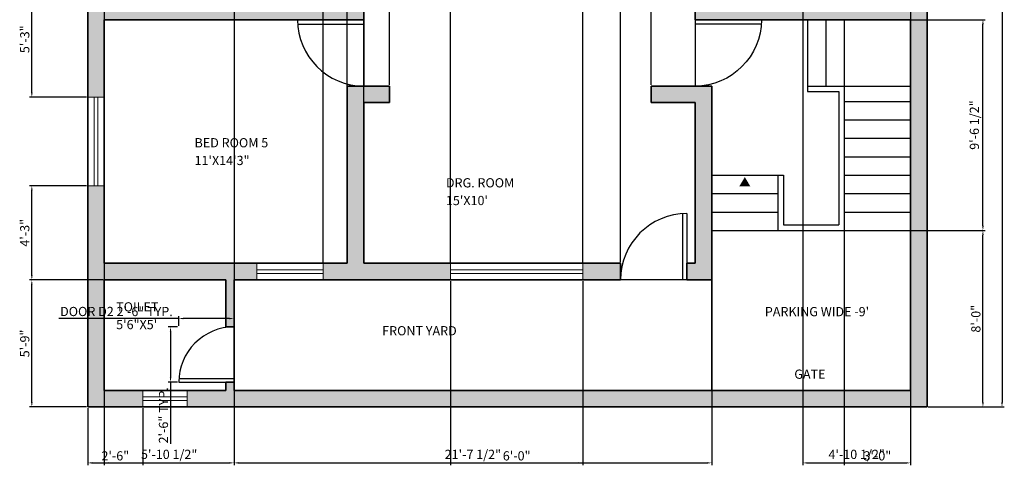
# Model space of a CAD drawing. Units: inches. Extents: x 2263 to 2802, y 2658 to 3310.
# Tile 1 of 3: x 2267 to 2802, y 2658 to 2902. Entities that reach past the tile are written whole.
import ezdxf

# ---------------------------------------------------------------- set-up
doc = ezdxf.new("R2010")
doc.units = ezdxf.units.IN
doc.header["$LTSCALE"] = 0.3
for name, color, linetype, lineweight in [('A-ANNO-DIMS', 2, 'Continuous', 18), ('A-ANNO-TEXT', 7, 'Continuous', 18), ('A-AREA-IDEN', 7, 'Continuous', 18), ('A-DOOR', 3, 'Continuous', 25), ('A-FLOR-STRS', 7, 'Continuous', 25), ('A-GLAZ', 4, 'Continuous', 18), ('A-WALL', 7, 'Continuous', 35)]:
    doc.layers.add(name, color=color, linetype=linetype, lineweight=lineweight)
doc.layers.add('A-WALL-PATT', color=18, linetype='Continuous', lineweight=13, true_color=0x000000)
doc.styles.get("Standard").update_dxf_attribs({"font": 'calibri.ttf', "height": 5})
doc.dimstyles.new('ISO-25', dxfattribs={"dimtxt": 5, "dimasz": 2.5, "dimexe": 1.25, "dimexo": 0.625, "dimtad": 1, "dimlunit": 3, "dimtxsty": 'Standard', "dimcen": 2.5, "dimadec": 0, "dimazin": 0, "dimtfac": 1, "dimtmove": 0, "dimatfit": 3, "dimfxl": 1, "dimarcsym": 0})

# ---------------------------------------------------------------- blocks, each defined once
blk = doc.blocks.new('*D2')
at = {"layer": 'A-ANNO-DIMS', "color": 0, "lineweight": -2, "transparency": 16777216}
for p, q in [((2761.03, 3268.27), (2802.38, 3268.27)), ((2801.13, 3265.77), (2801.13, 2694.77)), ((2761.03, 2692.27), (2802.38, 2692.27))]:
    blk.add_line(p, q, dxfattribs=at)
at = {"layer": 'A-ANNO-DIMS', "color": 0, "lineweight": -3, "transparency": 16777216}
for points in [[(2800.71, 3265.77), (2801.54, 3265.77), (2801.13, 3268.27)], [(2800.71, 2694.77), (2801.54, 2694.77), (2801.13, 2692.27)]]:
    blk.add_solid(points, dxfattribs=at)
at = {"layer": 'Defpoints', "color": 0, "lineweight": -3, "transparency": 16777216}
for p in [(2760.41, 3268.27), (2760.41, 2692.27), (2801.13, 2692.27)]:
    blk.add_point(p, dxfattribs=at)
at = {"layer": 'A-ANNO-DIMS', "color": 0, "transparency": 16777216, "insert": (2797.94, 2980.27), "char_height": 5, "attachment_point": 5, "rotation": 90}
blk.add_mtext("48'", dxfattribs=at)
blk = doc.blocks.new('DOOR-SWING-36')
for p, q in [((0, 0), (0, 36)), ((35.92, 2.4), (0, 2.4)), ((36, 0), (0, 0))]:
    blk.add_line(p, q)
blk.add_arc((0, 0), 36, 0, 90)
blk = doc.blocks.new('DOOR-SWING-30')
for p, q in [((30, 0), (0, 0)), ((0, 0), (0, -30)), ((29.93, -2), (0, -2))]:
    blk.add_line(p, q)
blk.add_arc((0, 0), 30, 270, 0)
blk = doc.blocks.new('WIN-24')
for p, q in [((0, 0), (0, -24)), ((9, 0), (0, 0)), ((3.5, 0), (3.5, -24)), ((5.5, 0), (5.5, -24)), ((9, -24), (9, 0)), ((0, -24), (9, -24))]:
    blk.add_line(p, q)
blk = doc.blocks.new('WIN-36')
for p, q in [((0, 36), (-9, 36)), ((-9, 36), (-9, 0)), ((-5.5, 0), (-5.5, 36)), ((-3.5, 0), (-3.5, 36)), ((0, 0), (0, 36)), ((-9, 0), (0, 0))]:
    blk.add_line(p, q)
blk = doc.blocks.new('WIN-48')
for p, q in [((0, 48), (-9, 48)), ((-9, 48), (-9, 0)), ((-5.5, 0), (-5.5, 48)), ((-3.5, 0), (-3.5, 48)), ((0, 0), (0, 48)), ((-9, 0), (0, 0))]:
    blk.add_line(p, q)
blk = doc.blocks.new('*D11')
at = {"layer": 'A-ANNO-DIMS', "color": 0, "lineweight": -2, "transparency": 16777216}
for p, q in [((2353.91, 2740.27), (2288.64, 2740.27)), ((2353.91, 2736.4), (2353.91, 2741.52)), ((2381.41, 2740.27), (2356.41, 2740.27)), ((2383.91, 2736.4), (2383.91, 2741.52))]:
    blk.add_line(p, q, dxfattribs=at)
at = {"layer": 'A-ANNO-DIMS', "color": 0, "lineweight": -3, "transparency": 16777216}
for points in [[(2356.41, 2740.69), (2356.41, 2739.86), (2353.91, 2740.27)], [(2381.41, 2740.69), (2381.41, 2739.86), (2383.91, 2740.27)]]:
    blk.add_solid(points, dxfattribs=at)
at = {"layer": 'Defpoints', "color": 0, "lineweight": -3, "transparency": 16777216}
for p in [(2353.91, 2740.27), (2353.91, 2735.77), (2383.91, 2735.77)]:
    blk.add_point(p, dxfattribs=at)
at = {"layer": 'A-ANNO-DIMS', "color": 0, "transparency": 16777216, "insert": (2320.02, 2743.46), "char_height": 5, "attachment_point": 5}
blk.add_mtext('DOOR D2 2\'-6" TYP.', dxfattribs=at)
blk = doc.blocks.new('*D12')
at = {"layer": 'A-ANNO-DIMS', "color": 0, "lineweight": -2, "transparency": 16777216}
for p, q in [((2353.28, 2735.77), (2348.16, 2735.77)), ((2349.41, 2733.27), (2349.41, 2708.27)), ((2353.28, 2705.77), (2348.16, 2705.77)), ((2349.41, 2705.77), (2349.41, 2672.23))]:
    blk.add_line(p, q, dxfattribs=at)
at = {"layer": 'A-ANNO-DIMS', "color": 0, "lineweight": -3, "transparency": 16777216}
for points in [[(2348.99, 2733.27), (2349.83, 2733.27), (2349.41, 2735.77)], [(2348.99, 2708.27), (2349.83, 2708.27), (2349.41, 2705.77)]]:
    blk.add_solid(points, dxfattribs=at)
at = {"layer": 'Defpoints', "color": 0, "lineweight": -3, "transparency": 16777216}
for p in [(2353.91, 2735.77), (2349.41, 2705.77), (2353.91, 2705.77)]:
    blk.add_point(p, dxfattribs=at)
at = {"layer": 'A-ANNO-DIMS', "color": 0, "transparency": 16777216, "insert": (2346.22, 2687.75), "char_height": 5, "attachment_point": 5, "rotation": 90}
blk.add_mtext('2\'-6" TYP.', dxfattribs=at)
blk = doc.blocks.new('*D21')
at = {"layer": 'A-ANNO-DIMS', "color": 0, "lineweight": -2, "transparency": 16777216}
for p, q in [((2312.78, 2761.27), (2272.81, 2761.27)), ((2274.06, 2694.77), (2274.06, 2758.77)), ((2303.78, 2692.27), (2272.81, 2692.27))]:
    blk.add_line(p, q, dxfattribs=at)
at = {"layer": 'A-ANNO-DIMS', "color": 0, "lineweight": -3, "transparency": 16777216}
for points in [[(2273.64, 2758.77), (2274.48, 2758.77), (2274.06, 2761.27)], [(2273.64, 2694.77), (2274.48, 2694.77), (2274.06, 2692.27)]]:
    blk.add_solid(points, dxfattribs=at)
at = {"layer": 'Defpoints', "color": 0, "lineweight": -3, "transparency": 16777216}
for p in [(2274.06, 2761.27), (2313.41, 2761.27), (2304.41, 2692.27)]:
    blk.add_point(p, dxfattribs=at)
at = {"layer": 'A-ANNO-DIMS', "color": 0, "transparency": 16777216, "insert": (2270.87, 2726.77), "char_height": 5, "attachment_point": 5, "rotation": 90}
blk.add_mtext('5\'-9"', dxfattribs=at)
blk = doc.blocks.new('*D22')
at = {"layer": 'A-ANNO-DIMS', "color": 0, "lineweight": -2, "transparency": 16777216}
for p, q in [((2303.78, 2812.37), (2272.81, 2812.37)), ((2274.06, 2763.77), (2274.06, 2809.87)), ((2312.78, 2761.27), (2272.81, 2761.27))]:
    blk.add_line(p, q, dxfattribs=at)
at = {"layer": 'A-ANNO-DIMS', "color": 0, "lineweight": -3, "transparency": 16777216}
for points in [[(2273.64, 2809.87), (2274.48, 2809.87), (2274.06, 2812.37)], [(2273.64, 2763.77), (2274.48, 2763.77), (2274.06, 2761.27)]]:
    blk.add_solid(points, dxfattribs=at)
at = {"layer": 'Defpoints', "color": 0, "lineweight": -3, "transparency": 16777216}
for p in [(2274.06, 2812.37), (2304.41, 2812.37), (2313.41, 2761.27)]:
    blk.add_point(p, dxfattribs=at)
at = {"layer": 'A-ANNO-DIMS', "color": 0, "transparency": 16777216, "insert": (2270.87, 2786.82), "char_height": 5, "attachment_point": 5, "rotation": 90}
blk.add_mtext('4\'-3"', dxfattribs=at)
blk = doc.blocks.new('*D23')
at = {"layer": 'A-ANNO-DIMS', "color": 0, "lineweight": -2, "transparency": 16777216}
for p, q in [((2303.78, 2923.37), (2272.81, 2923.37)), ((2274.06, 2862.87), (2274.06, 2920.87)), ((2303.78, 2860.37), (2272.81, 2860.37))]:
    blk.add_line(p, q, dxfattribs=at)
at = {"layer": 'A-ANNO-DIMS', "color": 0, "lineweight": -3, "transparency": 16777216}
for points in [[(2273.64, 2920.87), (2274.48, 2920.87), (2274.06, 2923.37)], [(2273.64, 2862.87), (2274.48, 2862.87), (2274.06, 2860.37)]]:
    blk.add_solid(points, dxfattribs=at)
at = {"layer": 'Defpoints', "color": 0, "lineweight": -3, "transparency": 16777216}
for p in [(2274.06, 2923.37), (2304.41, 2923.37), (2304.41, 2860.37)]:
    blk.add_point(p, dxfattribs=at)
at = {"layer": 'A-ANNO-DIMS', "color": 0, "transparency": 16777216, "insert": (2270.87, 2891.87), "char_height": 5, "attachment_point": 5, "rotation": 90}
blk.add_mtext('5\'-3"', dxfattribs=at)
blk = doc.blocks.new('*D26')
at = {"layer": 'A-ANNO-DIMS', "color": 0, "lineweight": -2, "transparency": 16777216}
for p, q in [((2304.41, 2691.65), (2304.41, 2660.67)), ((2334.41, 2691.65), (2334.41, 2660.67)), ((2306.91, 2661.92), (2331.91, 2661.92))]:
    blk.add_line(p, q, dxfattribs=at)
at = {"layer": 'A-ANNO-DIMS', "color": 0, "lineweight": -3, "transparency": 16777216}
for points in [[(2306.91, 2662.34), (2306.91, 2661.51), (2304.41, 2661.92)], [(2331.91, 2662.34), (2331.91, 2661.51), (2334.41, 2661.92)]]:
    blk.add_solid(points, dxfattribs=at)
at = {"layer": 'Defpoints', "color": 0, "lineweight": -3, "transparency": 16777216}
for p in [(2304.41, 2692.27), (2334.41, 2692.27), (2334.41, 2661.92)]:
    blk.add_point(p, dxfattribs=at)
at = {"layer": 'A-ANNO-DIMS', "color": 0, "transparency": 16777216, "insert": (2319.41, 2665.11), "char_height": 5, "attachment_point": 5}
blk.add_mtext('2\'-6"', dxfattribs=at)
blk = doc.blocks.new('*D27')
at = {"layer": 'A-ANNO-DIMS', "color": 0, "lineweight": -2, "transparency": 16777216}
for p, q in [((2383.91, 2700.65), (2383.91, 2660.67)), ((2643.41, 2700.65), (2643.41, 2660.67)), ((2386.41, 2661.92), (2640.91, 2661.92))]:
    blk.add_line(p, q, dxfattribs=at)
at = {"layer": 'A-ANNO-DIMS', "color": 0, "lineweight": -3, "transparency": 16777216}
for points in [[(2386.41, 2662.34), (2386.41, 2661.51), (2383.91, 2661.92)], [(2640.91, 2662.34), (2640.91, 2661.51), (2643.41, 2661.92)]]:
    blk.add_solid(points, dxfattribs=at)
at = {"layer": 'Defpoints', "color": 0, "lineweight": -3, "transparency": 16777216}
for p in [(2383.91, 2701.27), (2643.41, 2701.27), (2643.41, 2661.92)]:
    blk.add_point(p, dxfattribs=at)
at = {"layer": 'A-ANNO-DIMS', "color": 0, "transparency": 16777216, "insert": (2513.66, 2665.91), "char_height": 5, "attachment_point": 5}
blk.add_mtext('21\'-7 1/2"', dxfattribs=at)
blk = doc.blocks.new('*D28')
at = {"layer": 'A-ANNO-DIMS', "color": 0, "lineweight": -2, "transparency": 16777216}
for p, q in [((2501.46, 2760.65), (2501.46, 2660.67)), ((2573.46, 2760.65), (2573.46, 2660.67)), ((2503.96, 2661.92), (2570.96, 2661.92))]:
    blk.add_line(p, q, dxfattribs=at)
at = {"layer": 'A-ANNO-DIMS', "color": 0, "lineweight": -3, "transparency": 16777216}
for points in [[(2503.96, 2662.34), (2503.96, 2661.51), (2501.46, 2661.92)], [(2570.96, 2662.34), (2570.96, 2661.51), (2573.46, 2661.92)]]:
    blk.add_solid(points, dxfattribs=at)
at = {"layer": 'Defpoints', "color": 0, "lineweight": -3, "transparency": 16777216}
for p in [(2501.46, 2761.27), (2573.46, 2761.27), (2573.46, 2661.92)]:
    blk.add_point(p, dxfattribs=at)
at = {"layer": 'A-ANNO-DIMS', "color": 0, "transparency": 16777216, "insert": (2537.46, 2665.11), "char_height": 5, "attachment_point": 5}
blk.add_mtext('6\'-0"', dxfattribs=at)
blk = doc.blocks.new('*D29')
at = {"layer": 'A-ANNO-DIMS', "color": 0, "lineweight": -2, "transparency": 16777216}
for p, q in [((2454.41, 2770.9), (2454.41, 3299.87)), ((2456.91, 3298.62), (2498.96, 3298.62)), ((2501.46, 2770.9), (2501.46, 3299.87))]:
    blk.add_line(p, q, dxfattribs=at)
at = {"layer": 'A-ANNO-DIMS', "color": 0, "lineweight": -3, "transparency": 16777216}
for points in [[(2456.91, 3299.04), (2456.91, 3298.21), (2454.41, 3298.62)], [(2498.96, 3299.04), (2498.96, 3298.21), (2501.46, 3298.62)]]:
    blk.add_solid(points, dxfattribs=at)
at = {"layer": 'Defpoints', "color": 0, "lineweight": -3, "transparency": 16777216}
for p in [(2501.46, 3298.62), (2454.41, 2770.27), (2501.46, 2770.27)]:
    blk.add_point(p, dxfattribs=at)
at = {"layer": 'A-ANNO-DIMS', "color": 0, "transparency": 16777216, "insert": (2477.93, 3301.81), "char_height": 5, "attachment_point": 5}
blk.add_mtext('3\'-11"', dxfattribs=at)
blk = doc.blocks.new('*D30')
at = {"layer": 'A-ANNO-DIMS', "color": 0, "lineweight": -2, "transparency": 16777216}
for p, q in [((2573.46, 2770.9), (2573.46, 3299.87)), ((2575.96, 3298.62), (2591.41, 3298.62)), ((2593.91, 2770.9), (2593.91, 3299.87)), ((2593.91, 3298.62), (2624.49, 3298.62))]:
    blk.add_line(p, q, dxfattribs=at)
at = {"layer": 'A-ANNO-DIMS', "color": 0, "lineweight": -3, "transparency": 16777216}
for points in [[(2575.96, 3299.04), (2575.96, 3298.21), (2573.46, 3298.62)], [(2591.41, 3299.04), (2591.41, 3298.21), (2593.91, 3298.62)]]:
    blk.add_solid(points, dxfattribs=at)
at = {"layer": 'Defpoints', "color": 0, "lineweight": -3, "transparency": 16777216}
for p in [(2593.91, 3298.62), (2573.46, 2770.27), (2593.91, 2770.27)]:
    blk.add_point(p, dxfattribs=at)
at = {"layer": 'A-ANNO-DIMS', "color": 0, "transparency": 16777216, "insert": (2610.45, 3302.61), "char_height": 5, "attachment_point": 5}
blk.add_mtext('1\'-8 1/2"', dxfattribs=at)
blk = doc.blocks.new('*D31')
at = {"layer": 'A-ANNO-DIMS', "color": 0, "lineweight": -2, "transparency": 16777216}
for p, q in [((2432.25, 2770.9), (2432.25, 3299.87)), ((2434.75, 3298.62), (2442.91, 3298.62)), ((2445.41, 2770.9), (2445.41, 3299.87)), ((2445.41, 3298.62), (2463.19, 3298.62))]:
    blk.add_line(p, q, dxfattribs=at)
at = {"layer": 'A-ANNO-DIMS', "color": 0, "lineweight": -3, "transparency": 16777216}
for points in [[(2434.75, 3299.04), (2434.75, 3298.21), (2432.25, 3298.62)], [(2442.91, 3299.04), (2442.91, 3298.21), (2445.41, 3298.62)]]:
    blk.add_solid(points, dxfattribs=at)
at = {"layer": 'Defpoints', "color": 0, "lineweight": -3, "transparency": 16777216}
for p in [(2445.41, 3298.62), (2432.25, 2770.27), (2445.41, 2770.27)]:
    blk.add_point(p, dxfattribs=at)
at = {"layer": 'A-ANNO-DIMS', "color": 0, "transparency": 16777216, "insert": (2455.55, 3301.75), "char_height": 5, "attachment_point": 5}
blk.add_mtext('1\'-1"', dxfattribs=at)
blk = doc.blocks.new('*D32')
at = {"layer": 'A-ANNO-DIMS', "color": 0, "lineweight": -2, "transparency": 16777216}
for p, q in [((2715.41, 2787.47), (2715.41, 2660.67)), ((2751.41, 2787.47), (2751.41, 2660.67)), ((2717.91, 2661.92), (2748.91, 2661.92))]:
    blk.add_line(p, q, dxfattribs=at)
at = {"layer": 'A-ANNO-DIMS', "color": 0, "lineweight": -3, "transparency": 16777216}
for points in [[(2717.91, 2662.34), (2717.91, 2661.51), (2715.41, 2661.92)], [(2748.91, 2662.34), (2748.91, 2661.51), (2751.41, 2661.92)]]:
    blk.add_solid(points, dxfattribs=at)
at = {"layer": 'Defpoints', "color": 0, "lineweight": -3, "transparency": 16777216}
for p in [(2715.41, 2788.1), (2751.41, 2788.1), (2751.41, 2661.92)]:
    blk.add_point(p, dxfattribs=at)
at = {"layer": 'A-ANNO-DIMS', "color": 0, "transparency": 16777216, "insert": (2733.41, 2665.11), "char_height": 5, "attachment_point": 5}
blk.add_mtext('3\'-0"', dxfattribs=at)
blk = doc.blocks.new('*D36')
at = {"layer": 'A-ANNO-DIMS', "color": 0, "lineweight": -2, "transparency": 16777216}
for p, q in [((2752.03, 2788.1), (2792.01, 2788.1)), ((2790.76, 2694.77), (2790.76, 2785.6)), ((2761.03, 2692.27), (2792.01, 2692.27))]:
    blk.add_line(p, q, dxfattribs=at)
at = {"layer": 'A-ANNO-DIMS', "color": 0, "lineweight": -3, "transparency": 16777216}
for points in [[(2790.34, 2785.6), (2791.18, 2785.6), (2790.76, 2788.1)], [(2790.34, 2694.77), (2791.18, 2694.77), (2790.76, 2692.27)]]:
    blk.add_solid(points, dxfattribs=at)
at = {"layer": 'Defpoints', "color": 0, "lineweight": -3, "transparency": 16777216}
for p in [(2751.41, 2788.1), (2790.76, 2788.1), (2760.41, 2692.27)]:
    blk.add_point(p, dxfattribs=at)
at = {"layer": 'A-ANNO-DIMS', "color": 0, "transparency": 16777216, "insert": (2787.57, 2740.18), "char_height": 5, "attachment_point": 5, "rotation": 90}
blk.add_mtext('8\'-0"', dxfattribs=at)
blk = doc.blocks.new('*D37')
at = {"layer": 'A-ANNO-DIMS', "color": 0, "lineweight": -2, "transparency": 16777216}
for p, q in [((2752.03, 2902.48), (2792.01, 2902.48)), ((2790.76, 2790.6), (2790.76, 2899.98)), ((2752.03, 2788.1), (2792.01, 2788.1))]:
    blk.add_line(p, q, dxfattribs=at)
at = {"layer": 'A-ANNO-DIMS', "color": 0, "lineweight": -3, "transparency": 16777216}
for points in [[(2790.34, 2899.98), (2791.18, 2899.98), (2790.76, 2902.48)], [(2790.34, 2790.6), (2791.18, 2790.6), (2790.76, 2788.1)]]:
    blk.add_solid(points, dxfattribs=at)
at = {"layer": 'Defpoints', "color": 0, "lineweight": -3, "transparency": 16777216}
for p in [(2751.41, 2902.48), (2790.76, 2902.48), (2751.41, 2788.1)]:
    blk.add_point(p, dxfattribs=at)
at = {"layer": 'A-ANNO-DIMS', "color": 0, "transparency": 16777216, "insert": (2786.77, 2845.29), "char_height": 5, "attachment_point": 5, "rotation": 90}
blk.add_mtext('9\'-6 1/2"', dxfattribs=at)
blk = doc.blocks.new('*D42')
at = {"layer": 'A-ANNO-DIMS', "color": 0, "lineweight": -2, "transparency": 16777216}
for p, q in [((2468.29, 2867.1), (2468.29, 3299.87)), ((2470.79, 3298.62), (2608, 3298.62)), ((2610.5, 2867.1), (2610.5, 3299.87))]:
    blk.add_line(p, q, dxfattribs=at)
at = {"layer": 'A-ANNO-DIMS', "color": 0, "lineweight": -3, "transparency": 16777216}
for points in [[(2470.79, 3299.04), (2470.79, 3298.21), (2468.29, 3298.62)], [(2608, 3299.04), (2608, 3298.21), (2610.5, 3298.62)]]:
    blk.add_solid(points, dxfattribs=at)
at = {"layer": 'Defpoints', "color": 0, "lineweight": -3, "transparency": 16777216}
for p in [(2610.5, 3298.62), (2468.29, 2866.48), (2610.5, 2866.48)]:
    blk.add_point(p, dxfattribs=at)
at = {"layer": 'A-ANNO-DIMS', "color": 0, "transparency": 16777216, "insert": (2539.4, 3301.81), "char_height": 5, "attachment_point": 5}
blk.add_mtext('11\'-10"', dxfattribs=at)
blk = doc.blocks.new('*D43')
at = {"layer": 'A-ANNO-DIMS', "color": 0, "lineweight": -2, "transparency": 16777216}
for p, q in [((2383.91, 3114.65), (2383.91, 2660.67)), ((2313.41, 3105.65), (2313.41, 2660.67)), ((2315.91, 2661.92), (2381.41, 2661.92))]:
    blk.add_line(p, q, dxfattribs=at)
at = {"layer": 'A-ANNO-DIMS', "color": 0, "lineweight": -3, "transparency": 16777216}
for points in [[(2315.91, 2662.34), (2315.91, 2661.51), (2313.41, 2661.92)], [(2381.41, 2662.34), (2381.41, 2661.51), (2383.91, 2661.92)]]:
    blk.add_solid(points, dxfattribs=at)
at = {"layer": 'Defpoints', "color": 0, "lineweight": -3, "transparency": 16777216}
for p in [(2383.91, 3115.27), (2313.41, 3106.27), (2383.91, 2661.92)]:
    blk.add_point(p, dxfattribs=at)
at = {"layer": 'A-ANNO-DIMS', "color": 0, "transparency": 16777216, "insert": (2348.66, 2665.91), "char_height": 5, "attachment_point": 5}
blk.add_mtext('5\'-10 1/2"', dxfattribs=at)
blk = doc.blocks.new('*D44')
at = {"layer": 'A-ANNO-DIMS', "color": 0, "lineweight": -2, "transparency": 16777216}
for p, q in [((2692.91, 3114.65), (2692.91, 2660.67)), ((2751.41, 3105.65), (2751.41, 2660.67)), ((2695.41, 2661.92), (2748.91, 2661.92))]:
    blk.add_line(p, q, dxfattribs=at)
at = {"layer": 'A-ANNO-DIMS', "color": 0, "lineweight": -3, "transparency": 16777216}
for points in [[(2695.41, 2662.34), (2695.41, 2661.51), (2692.91, 2661.92)], [(2748.91, 2662.34), (2748.91, 2661.51), (2751.41, 2661.92)]]:
    blk.add_solid(points, dxfattribs=at)
at = {"layer": 'Defpoints', "color": 0, "lineweight": -3, "transparency": 16777216}
for p in [(2692.91, 3115.27), (2751.41, 3106.27), (2751.41, 2661.92)]:
    blk.add_point(p, dxfattribs=at)
at = {"layer": 'A-ANNO-DIMS', "color": 0, "transparency": 16777216, "insert": (2722.16, 2665.91), "char_height": 5, "attachment_point": 5}
blk.add_mtext('4\'-10 1/2"', dxfattribs=at)

msp = doc.modelspace()

# ---------------------------------------------------------------- hatches: boundary and pattern name
at = {"layer": 'A-WALL-PATT'}
h = msp.add_hatch(color=256, dxfattribs=at)
h.dxf.hatch_style = 1
h.paths.add_polyline_path([(2454.409, 2984.773), (2445.409, 2984.773), (2445.409, 2980.273), (2313.409, 2980.273), (2313.409, 3019.273), (2304.409, 3019.273), (2304.409, 2959.375), (2313.409, 2959.375), (2313.409, 2975.773), (2454.409, 2975.773)], flags=17)
h.paths.add_polyline_path([(2313.409, 2902.477), (2454.409, 2902.477), (2454.409, 2906.977), (2313.409, 2906.977), (2313.409, 2923.375), (2304.409, 2923.375), (2304.409, 2860.375), (2313.409, 2860.375)], flags=17)
h.paths.add_polyline_path([(2313.409, 2812.375), (2304.409, 2812.375), (2304.409, 2692.273), (2334.409, 2692.273), (2334.409, 2701.273), (2313.409, 2701.273), (2313.409, 2761.273), (2379.409, 2761.273), (2379.409, 2735.773), (2383.909, 2735.773), (2383.909, 2761.273), (2396.251, 2761.273), (2396.251, 2770.273), (2313.409, 2770.273)], flags=17)
h.paths.add_polyline_path([(2760.409, 3268.273), (2304.409, 3268.273), (2304.409, 3157.273), (2313.409, 3157.273), (2313.409, 3175.273), (2317.909, 3175.273), (2317.909, 3179.773), (2313.409, 3179.773), (2313.409, 3259.273), (2379.409, 3259.273), (2379.409, 3254.773), (2383.909, 3254.773), (2383.909, 3259.273), (2533.909, 3259.273), (2533.909, 3115.273), (2529.409, 3115.273), (2529.409, 3106.273), (2547.409, 3106.273), (2547.409, 3115.273), (2542.909, 3115.273), (2542.909, 3259.273), (2692.909, 3259.273), (2692.909, 3254.773), (2697.409, 3254.773), (2697.409, 3259.273), (2751.409, 3259.273), (2751.409, 3179.773), (2746.909, 3179.773), (2746.909, 3175.273), (2751.409, 3175.273), (2751.409, 3115.273), (2697.409, 3115.273), (2697.409, 3175.273), (2716.909, 3175.273), (2716.909, 3179.773), (2697.409, 3179.773), (2697.409, 3224.773), (2692.909, 3224.773), (2692.909, 3115.273), (2583.409, 3115.273), (2583.409, 3106.273), (2610.409, 3106.273), (2610.409, 3090.217), (2619.409, 3090.217), (2619.409, 3106.273), (2751.409, 3106.273), (2751.409, 2980.273), (2619.409, 2980.273), (2619.409, 2984.773), (2610.409, 2984.773), (2610.409, 2975.773), (2751.409, 2975.773), (2751.409, 2906.977), (2634.409, 2906.977), (2634.409, 2902.477), (2670.409, 2902.477), (2751.409, 2902.477), (2751.409, 2701.273), (2383.909, 2701.273), (2383.909, 2705.773), (2379.409, 2705.773), (2379.409, 2701.273), (2358.409, 2701.273), (2358.409, 2692.273), (2760.409, 2692.273)])
h.paths.add_polyline_path([(2501.459, 2770.273), (2454.409, 2770.273), (2454.409, 2857.477), (2468.293, 2857.477), (2468.293, 2866.477), (2445.409, 2866.477), (2445.409, 2770.273), (2432.251, 2770.273), (2432.251, 2761.273), (2501.459, 2761.273)], flags=17)
h.paths.add_polyline_path([(2593.909, 2770.273), (2573.459, 2770.273), (2573.459, 2761.273), (2593.909, 2761.273)], flags=17)
h.paths.add_polyline_path([(2643.409, 2866.477), (2610.501, 2866.477), (2610.501, 2857.477), (2634.409, 2857.477), (2634.409, 2770.273), (2629.909, 2770.273), (2629.909, 2761.273), (2643.409, 2761.273)], flags=17)
h.paths.add_polyline_path([(2643.409, 2930.977), (2634.409, 2930.977), (2634.409, 2906.977), (2643.409, 2906.977)], flags=17)
h.paths.add_polyline_path([(2454.409, 2930.977), (2445.409, 2930.977), (2445.409, 2906.977), (2454.409, 2906.977)], flags=17)
h.paths.add_polyline_path([(2454.409, 3106.273), (2493.409, 3106.273), (2493.409, 3115.273), (2383.909, 3115.273), (2383.909, 3224.773), (2379.409, 3224.773), (2379.409, 3179.773), (2347.909, 3179.773), (2347.909, 3175.273), (2379.409, 3175.273), (2379.409, 3115.273), (2313.409, 3115.273), (2313.409, 3133.273), (2304.409, 3133.273), (2304.409, 3067.273), (2313.409, 3067.273), (2313.409, 3106.273), (2445.409, 3106.273), (2445.409, 3020.773), (2454.409, 3020.773)], flags=17)
h.paths.add_polyline_path([(2619.409, 3054.217), (2610.409, 3054.217), (2610.409, 3020.773), (2619.409, 3020.773)], flags=17)

# ---------------------------------------------------------------- linework, layer by layer
at = {"layer": 'A-FLOR-STRS'}
for p, q in [((2695.409, 2902.477), (2695.409, 2863.477)), ((2705.409, 2902.477), (2705.409, 2866.477)), ((2715.409, 2902.477), (2715.409, 2788.095)), ((2695.409, 2866.477), (2751.409, 2866.477)), ((2695.409, 2863.477), (2712.409, 2863.477)), ((2712.409, 2863.477), (2712.409, 2791.095)), ((2715.409, 2858.095), (2751.409, 2858.095)), ((2715.409, 2848.095), (2751.409, 2848.095)), ((2715.409, 2838.095), (2751.409, 2838.095)), ((2715.409, 2828.095), (2751.409, 2828.095)), ((2643.409, 2818.095), (2682.409, 2818.095)), ((2679.409, 2818.095), (2679.409, 2788.095)), ((2682.409, 2818.095), (2682.409, 2791.095)), ((2715.409, 2818.095), (2751.409, 2818.095)), ((2643.409, 2808.095), (2679.409, 2808.095)), ((2715.409, 2808.095), (2751.409, 2808.095)), ((2643.409, 2798.095), (2679.409, 2798.095)), ((2715.409, 2798.095), (2751.409, 2798.095)), ((2643.409, 2788.095), (2751.409, 2788.095)), ((2682.409, 2791.095), (2712.409, 2791.095))]:
    msp.add_line(p, q, dxfattribs=at)
for points in [[(2695.409, 2884.477, 0, 0, 0), (2733.409, 2884.477, 0, 0, 0), (2733.409, 2753.71, 0, 0, 0), (2661.409, 2753.71, 0, 0, 0), (2661.409, 2812.013, 0, 6, 0), (2661.409, 2812.013, 6, 6, 0)], [(2661.409, 2812.013, 6, 0, 0), (2661.409, 2817.031, 0, 0, 0)]]:
    msp.add_lwpolyline(points, format="xyseb", dxfattribs=at)
at = {"layer": 'A-GLAZ'}
for p, q in [((2573.459, 2770.273), (2501.459, 2770.273)), ((2501.459, 2770.273), (2501.459, 2761.273)), ((2573.459, 2766.773), (2501.459, 2766.773)), ((2573.459, 2761.273), (2573.459, 2770.273)), ((2573.459, 2764.773), (2501.459, 2764.773)), ((2501.459, 2761.273), (2573.459, 2761.273))]:
    msp.add_line(p, q, dxfattribs=at)
at = {"layer": 'A-WALL'}
for p, q in [((2304.409, 2692.273), (2304.409, 3268.273)), ((2760.409, 3268.273), (2760.409, 2692.273)), ((2454.409, 2906.977), (2454.409, 2902.477)), ((2634.409, 2906.977), (2634.409, 2902.477)), ((2313.409, 2902.477), (2454.409, 2902.477)), ((2313.409, 2770.273), (2313.409, 2902.477)), ((2634.409, 2902.477), (2751.409, 2902.477)), ((2751.409, 2902.477), (2751.409, 2701.273)), ((2445.409, 2770.273), (2445.409, 2866.477)), ((2445.409, 2866.477), (2468.293, 2866.477)), ((2468.293, 2866.477), (2468.293, 2857.477)), ((2610.501, 2866.477), (2610.501, 2857.477)), ((2610.501, 2866.477), (2643.409, 2866.477)), ((2634.409, 2866.477), (2643.409, 2866.477)), ((2643.409, 2866.477), (2643.409, 2701.273)), ((2454.409, 2857.477), (2468.293, 2857.477)), ((2454.409, 2857.477), (2454.409, 2770.273)), ((2610.501, 2857.477), (2634.409, 2857.477)), ((2634.409, 2857.477), (2634.409, 2770.273)), ((2445.409, 2770.273), (2313.409, 2770.273)), ((2593.909, 2770.273), (2454.409, 2770.273)), ((2593.909, 2770.273), (2593.909, 2761.273)), ((2634.409, 2770.273), (2629.909, 2770.273)), ((2629.909, 2770.273), (2629.909, 2761.273)), ((2313.409, 2701.273), (2313.409, 2761.273)), ((2379.409, 2761.273), (2313.409, 2761.273)), ((2379.409, 2735.773), (2379.409, 2761.273)), ((2383.909, 2735.773), (2383.909, 2761.273)), ((2593.909, 2761.273), (2383.909, 2761.273)), ((2643.409, 2761.273), (2629.909, 2761.273)), ((2379.409, 2735.773), (2383.909, 2735.773)), ((2379.409, 2701.273), (2379.409, 2705.773)), ((2379.409, 2705.773), (2383.909, 2705.773)), ((2383.909, 2701.273), (2383.909, 2705.773)), ((2379.409, 2701.273), (2313.409, 2701.273)), ((2751.409, 2701.273), (2383.909, 2701.273)), ((2760.409, 2692.273), (2304.409, 2692.273))]:
    msp.add_line(p, q, dxfattribs=at)

# ---------------------------------------------------------------- block references
at = {"layer": 'A-DOOR'}
for name, p, rotation in [('DOOR-SWING-36', (2454.409, 2902.477), 180), ('DOOR-SWING-36', (2629.909, 2761.273), 89.9999999999844), ('DOOR-SWING-30', (2383.909, 2705.773), 180)]:
    msp.add_blockref(name, p, dxfattribs=dict(at, rotation=rotation))
at = {"layer": 'A-DOOR', "extrusion": (0, 0, -1), "zscale": -1, "rotation": 180}
msp.add_blockref('DOOR-SWING-36', (-2634.409, 2902.477), dxfattribs=at)
at = {"layer": 'A-GLAZ'}
msp.add_blockref('WIN-48', (2313.409, 2812.375), dxfattribs=at)
for name, p, rotation in [('WIN-36', (2432.251, 2770.273), 90.00000000000102), ('WIN-24', (2334.409, 2692.273), 89.99999999999666)]:
    msp.add_blockref(name, p, dxfattribs=dict(at, rotation=rotation))

# ---------------------------------------------------------------- texts
at = {"layer": 'A-ANNO-TEXT'}
msp.add_text('GATE', height=5, dxfattribs=at).set_placement((2688.291, 2707.586))
at = {"layer": 'A-AREA-IDEN'}
for s, p in [('BED ROOM 5', (2362.462, 2833.203)), ('11\'X14\'3"', (2362.462, 2823.588)), ('DRG. ROOM', (2499.02, 2811.455)), ("15'X10'", (2499.02, 2801.84)), ('TOILET', (2319.867, 2744.12)), ("PARKING WIDE -9'", (2672.297, 2741.529)), ('5\'6"X5\'', (2319.867, 2734.505)), ('FRONT YARD', (2464.403, 2731.161))]:
    msp.add_text(s, height=5, dxfattribs=at).set_placement(p)

# ---------------------------------------------------------------- dimensions: what is measured, and where the dimension line sits
at = {"layer": 'A-ANNO-DIMS'}
for base, p1, p2, picture, middle in [((2593.9094, 3298.6226), (2573.459, 2770.2726), (2593.9094, 2770.2726), '*D30', (2610.4517, 3302.6149)), ((2445.409, 3298.623), (2432.251, 2770.273), (2445.409, 2770.273), '*D31', (2455.548, 3301.753)), ((2501.459, 3298.6226), (2454.4094, 2770.2726), (2501.459, 2770.2726), '*D29', (2477.9342, 3301.8092)), ((2610.501, 3298.623), (2468.293, 2866.477), (2610.501, 2866.477), '*D42', (2539.397, 3301.809)), ((2383.909, 2661.923), (2313.409, 3106.273), (2383.909, 3115.273), '*D43', (2348.659, 2665.915)), ((2751.409, 2661.923), (2692.909, 3115.273), (2751.409, 3106.273), '*D44', (2722.159, 2665.915)), ((2751.409, 2661.923), (2715.409, 2788.095), (2751.409, 2788.095), '*D32', (2733.409, 2665.109)), ((2573.459, 2661.923), (2501.459, 2761.273), (2573.459, 2761.273), '*D28', (2537.459, 2665.109)), ((2643.409, 2661.923), (2383.909, 2701.273), (2643.409, 2701.273), '*D27', (2513.659, 2665.915)), ((2334.409, 2661.923), (2304.409, 2692.273), (2334.409, 2692.273), '*D26', (2319.409, 2665.109))]:
    dim = msp.add_linear_dim(base=base, p1=p1, p2=p2, dimstyle='ISO-25', override={"dimdec": 1, "dimlfac": 1, "dimrnd": 0, "dimzin": 1, "dimdsep": 46, "dimlunit": 4, "dimfrac": 2}, dxfattribs=at)
    dim.commit()
    dim.dimension.update_dxf_attribs({"geometry": picture, "text_midpoint": middle})
for base, p1, p2, override, picture, middle in [((2801.125, 2692.273), (2760.409, 3268.273), (2760.409, 2692.273), {"dimclrd": 0, "dimclre": 0, "dimclrt": 0}, '*D2', (2797.939, 2980.273)), ((2274.059, 2923.375), (2304.409, 2860.375), (2304.409, 2923.375), {"dimdec": 1, "dimlfac": 1, "dimrnd": 0, "dimzin": 1, "dimdsep": 46, "dimlunit": 4, "dimfrac": 2}, '*D23', (2270.873, 2891.875)), ((2790.759, 2902.477), (2751.409, 2788.095), (2751.409, 2902.477), {"dimdec": 1, "dimlfac": 1, "dimrnd": 0, "dimzin": 1, "dimdsep": 46, "dimlunit": 4, "dimfrac": 2}, '*D37', (2786.767, 2845.286)), ((2274.059, 2812.375), (2313.409, 2761.273), (2304.409, 2812.375), {"dimdec": 1, "dimlfac": 1, "dimrnd": 0, "dimzin": 1, "dimdsep": 46, "dimlunit": 4, "dimfrac": 2}, '*D22', (2270.873, 2786.824)), ((2790.759, 2788.095), (2760.409, 2692.273), (2751.409, 2788.095), {"dimdec": 1, "dimlfac": 1, "dimrnd": 0, "dimzin": 1, "dimdsep": 46, "dimlunit": 4, "dimfrac": 2}, '*D36', (2787.573, 2740.184)), ((2274.059, 2761.273), (2304.409, 2692.273), (2313.409, 2761.273), {"dimdec": 1, "dimlfac": 1, "dimrnd": 0, "dimzin": 1, "dimdsep": 46, "dimlunit": 4, "dimfrac": 2}, '*D21', (2270.873, 2726.773))]:
    dim = msp.add_linear_dim(base=base, p1=p1, p2=p2, angle=90, dimstyle='ISO-25', override=override, dxfattribs=at)
    dim.commit()
    dim.dimension.update_dxf_attribs({"geometry": picture, "text_midpoint": middle})
for base, p1, p2, angle, text, picture, middle in [((2353.909, 2740.273), (2383.909, 2735.773), (2353.909, 2735.773), 180, 'DOOR D2 <> TYP.', '*D11', (2320.025, 2743.459)), ((2349.409, 2705.773), (2353.909, 2735.773), (2353.909, 2705.773), 270, '<> TYP.', '*D12', (2346.223, 2687.753))]:
    dim = msp.add_linear_dim(base=base, p1=p1, p2=p2, angle=angle, text=text, dimstyle='ISO-25', override={"dimdec": 1, "dimlfac": 1, "dimrnd": 0, "dimzin": 1, "dimdsep": 46, "dimlunit": 4, "dimfrac": 2}, dxfattribs=at)
    dim.commit()
    dim.dimension.update_dxf_attribs({"geometry": picture, "text_midpoint": middle})

doc.saveas('drawing.dxf')
